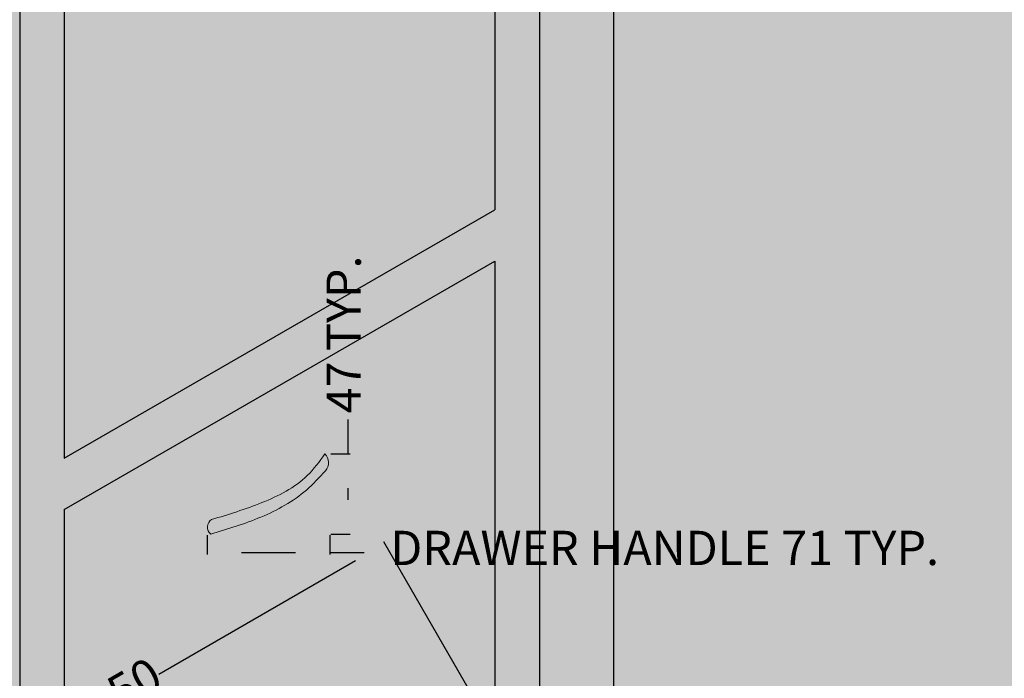
# Model space of a CAD drawing. Units: millimetres. Extents: x 78378 to 86415, y 148682 to 152721.
# Tile 8 of 18: x 79783 to 80358, y 149707 to 150092. Entities that reach past the tile are written whole.
import ezdxf

# ---------------------------------------------------------------- set-up
doc = ezdxf.new("R2010")
doc.units = ezdxf.units.MM
for name, color, linetype, lineweight in [('A-ANNO-DIMS', 2, 'Continuous', 18), ('A-FURN', 4, 'Continuous', 25), ('A-FURN-HRDW', 8, 'Continuous', 18), ('A-FURN-PATT', 32, 'Continuous', 13)]:
    doc.layers.add(name, color=color, linetype=linetype, lineweight=lineweight)
doc.styles.get("Standard").update_dxf_attribs({"font": 'arial.ttf'})
doc.dimstyles.new('ISO-25', dxfattribs={"dimtxt": 20, "dimasz": 20, "dimexe": 1.25, "dimexo": 0.625, "dimtad": 0, "dimdec": 1, "dimtxsty": 'Standard', "dimcen": 2.5, "dimadec": 0, "dimazin": 0, "dimtfac": 1, "dimtdec": 1, "dimtmove": 0, "dimatfit": 3, "dimfxl": 1, "dimarcsym": 0})

# ---------------------------------------------------------------- blocks, each defined once
blk = doc.blocks.new('HANDLE-DRAWER')
for centre, radius, start, end in [((63.38622997708444, 41.62154367045149), 7.231969022595942, 319.3237562697811, 44.69265733271547), ((5.163435732683865, 4.025219173752702), 5.172557027146686, 122.0794663418697, 231.0916038547452)]:
    blk.add_arc(centre, radius, start, end)
for points, knots in [([(2.416316796850878, 8.407990414794767), (12.22361058796001, 11.4080339887645), (31.81170594566225, 17.4000171857454), (55.97206586949582, 29.46692429189343), (65.30177131113433, 42.2784439569471), (68.52736162004294, 46.70781355843064)], [0, 0, 0, 0, 30.92804236988506, 61.77253950703249, 78.07166049105084, 78.07166049105084, 78.07166049105084, 78.07166049105084]), ([(1.914671141596045, 0.0001881390053313), (11.78696018195832, 2.942018891461464), (31.50487046795086, 8.817733694416148), (54.70585002572761, 21.54120260495396), (65.2835446695137, 33.01612223177024), (68.87098889380286, 36.90786192796077)], [0, 0, 0, 0, 30.92804236988506, 61.77253950704738, 77.60214595393334, 77.60214595393334, 77.60214595393334, 77.60214595393334])]:
    blk.add_open_spline(points, degree=3, knots=knots)
blk = doc.blocks.new('*D12')
at = {"layer": 'A-ANNO-DIMS', "color": 0, "lineweight": -2, "transparency": 16777216}
for p, q in [((79892.72448662344, 149790.980188139), (79892.72448662344, 149779.6412546455)), ((79964.1507099133, 149790.980188139), (79964.1507099133, 149779.6412546455)), ((79912.72448662344, 149780.8912546455), (79944.1507099133, 149780.8912546455)), ((79964.1507099133, 149780.8912546455), (79984.1507099133, 149780.8912546455))]:
    blk.add_line(p, q, dxfattribs=at)
at = {"layer": 'A-ANNO-DIMS', "color": 0, "transparency": 16777216}
for points in [[(79912.72448662344, 149784.2245879789), (79912.72448662344, 149777.5579213122), (79892.72448662344, 149780.8912546455)], [(79944.1507099133, 149784.2245879789), (79944.1507099133, 149777.5579213122), (79964.1507099133, 149780.8912546455)]]:
    blk.add_solid(points, dxfattribs=at)
at = {"layer": 'Defpoints', "color": 0, "transparency": 16777216}
for p in [(79892.72448662344, 149791.605188139), (79964.1507099133, 149791.605188139), (79964.1507099133, 149780.8912546455)]:
    blk.add_point(p, dxfattribs=at)
at = {"layer": 'A-ANNO-DIMS', "color": 0, "transparency": 16777216, "insert": (80159.47557348765, 149780.8912546455), "char_height": 20, "attachment_point": 5}
blk.add_mtext('DRAWER HANDLE 71 TYP.', dxfattribs=at)
blk = doc.blocks.new('*D13')
at = {"layer": 'A-ANNO-DIMS', "color": 0, "lineweight": -2, "transparency": 16777216}
for p, q in [((79974.86464340684, 149838.3128135585), (79974.86464340684, 149858.3128135585)), ((79964.77570991333, 149838.3128135585), (79976.11464340684, 149838.3128135585)), ((79974.86464340684, 149811.6051881391), (79974.86464340684, 149818.3128135585)), ((79964.77570991333, 149791.605188139), (79976.11464340684, 149791.605188139))]:
    blk.add_line(p, q, dxfattribs=at)
at = {"layer": 'A-ANNO-DIMS', "color": 0, "transparency": 16777216}
for points in [[(79971.5313100735, 149818.3128135585), (79978.19797674016, 149818.3128135585), (79974.86464340684, 149838.3128135585)], [(79971.5313100735, 149811.6051881391), (79978.19797674016, 149811.6051881391), (79974.86464340684, 149791.605188139)]]:
    blk.add_solid(points, dxfattribs=at)
at = {"layer": 'Defpoints', "color": 0, "transparency": 16777216}
for p in [(79964.15070991333, 149838.3128135585), (79974.86464340684, 149838.3128135585), (79964.15070991333, 149791.605188139)]:
    blk.add_point(p, dxfattribs=at)
at = {"layer": 'A-ANNO-DIMS', "color": 0, "transparency": 16777216, "insert": (79974.86464340687, 149908.0169404343), "char_height": 20, "attachment_point": 5, "rotation": 90}
blk.add_mtext('47 TYP.', dxfattribs=at)
blk = doc.blocks.new('*D22')
at = {"layer": 'A-ANNO-DIMS', "color": 0, "lineweight": -2, "transparency": 16777216}
for p, q in [((80086.091702, 149630.5489088773), (79995.77920202748, 149786.9747473883)), ((79979.08369395178, 149775.8922156335), (79864.48965899751, 149709.7313187051)), ((79710.61581902203, 149620.892215774), (79825.2098539763, 149687.0531127024)), ((79782.98281099998, 149455.5489088774), (79692.67031094636, 149611.9747475287))]:
    blk.add_line(p, q, dxfattribs=at)
at = {"layer": 'A-ANNO-DIMS', "color": 0, "transparency": 16777216}
for points in [[(79977.41702728512, 149778.7789669795), (79980.75036061846, 149773.0054642876), (79996.40420202748, 149785.8922156335)], [(79708.94915235537, 149623.7789671199), (79712.28248568872, 149618.005464428), (79693.29531094636, 149610.892215774)]]:
    blk.add_solid(points, dxfattribs=at)
at = {"layer": 'Defpoints', "color": 0, "transparency": 16777216}
for p in [(79996.40420202748, 149785.8922156335), (80086.404202, 149630.007643), (79783.29531099998, 149455.007643)]:
    blk.add_point(p, dxfattribs=at)
at = {"layer": 'A-ANNO-DIMS', "color": 0, "transparency": 16777216, "insert": (79844.84975648689, 149698.3922157038), "char_height": 20, "attachment_point": 5, "rotation": 30.000000000013433}
blk.add_mtext('350', dxfattribs=at)
blk = doc.blocks.new('*D32')
at = {"layer": 'A-ANNO-DIMS', "color": 0, "lineweight": -2, "transparency": 16777216}
for p, q in [((80086.404202, 150459.382643), (80086.404202, 148693.757643)), ((80692.621985, 150459.382643), (80692.621985, 148693.757643)), ((80106.404202, 148695.007643), (80355.19095843862, 148695.007643)), ((80672.621985, 148695.007643), (80423.8352285614, 148695.007643))]:
    blk.add_line(p, q, dxfattribs=at)
at = {"layer": 'A-ANNO-DIMS', "color": 0, "transparency": 16777216}
for points in [[(80106.404202, 148698.3409763333), (80106.404202, 148691.6743096666), (80086.404202, 148695.007643)], [(80672.621985, 148698.3409763333), (80672.621985, 148691.6743096666), (80692.621985, 148695.007643)]]:
    blk.add_solid(points, dxfattribs=at)
at = {"layer": 'Defpoints', "color": 0, "transparency": 16777216}
for p in [(80086.404202, 150460.007643), (80692.621985, 150460.007643), (80692.621985, 148695.007643)]:
    blk.add_point(p, dxfattribs=at)
at = {"layer": 'A-ANNO-DIMS', "color": 0, "transparency": 16777216, "insert": (80389.5130935, 148695.007643), "char_height": 20, "attachment_point": 5}
blk.add_mtext('606.2', dxfattribs=at)

msp = doc.modelspace()

# ---------------------------------------------------------------- hatches: boundary and pattern name
at = {"layer": 'A-FURN-PATT'}
h = msp.add_hatch(color=256, dxfattribs=at)
h.dxf.hatch_style = 1
h.paths.add_polyline_path([(80389.81355980314, 150935.1811176149), (80389.51309381555, 151105.0076434962), (80164.3464888316, 151105.0076434962), (79904.53886769625, 150955.0076434962), (79433.58476952511, 150683.1021681411), (79459.41281351625, 150662.3818050495), (79243.9048024148, 150537.9581968276), (79160.4069246431, 150518.167363956), (78839.3276210414, 150320.0076434962), (78579.51999990609, 150470.0076434961), (78570.85974586825, 150475.0076434961), (78570.85974586825, 150465.0076434962), (78570.85974586825, 149885.0076434961)])
h.paths.add_polyline_path([(80086.40420249099, 150460.0076434961), (79826.59658135568, 150610.0076434961), (78570.85974586825, 149885.0076434961), (78830.66736700358, 149735.0076434961)])
h.paths.add_polyline_path([(79540.80006404899, 150161.0556565937), (79217.39666007676, 149974.3386142535), (78980.9165707482, 150110.8704574853), (79304.31997472048, 150297.5874998256)], flags=16)
h.paths.add_polyline_path([(79506.15904789761, 150161.0556565937), (79217.39666007677, 149994.3386142535), (79015.55758689957, 150110.8704574853), (79304.31997472048, 150277.5874998256)], flags=0)
edge = h.paths.add_edge_path(flags=0)
edge.add_arc((79247.8635885932, 150177.154059363), 137.979927152229, 256.0025927560106, 293.5594108656914)
edge.add_arc((79240.76712928673, 150078.260535577), 68.08549769177299, 336.0991039681863, 387.369687653981)
edge.add_ellipse((79258.3073696606, 150109.4851683714), major_axis=(-42.62344506003415, -1.659142297571932), ratio=0.1604284291443649, start_angle=0, end_angle=179.0977278657225, ccw=False)
edge.add_arc((79285.21118690472, 150074.2509041072), 77.20964330046426, 155.1233103751286, 203.6557939001038)
edge = h.paths.add_edge_path(flags=0)
edge.add_ellipse((79258.69578401413, 150110.8297486024), major_axis=(-42.62344506003415, -1.659142297571932), ratio=0.1604284291443649, start_angle=350.6039411592706, end_angle=356.2289762200799)
edge.add_line((79219.16897707367, 150111.8937051806), (79218.32684768032, 150109.4140931549))
edge.add_arc((79262.46751974897, 150032.9602064517), 88.28134413732826, 112.39312291994881, 119.99999999999571, ccw=False)
h.paths.add_polyline_path([(79287.06250338514, 150086.9702731333, -0.247702064009433), (79288.19674658246, 150077.2955427019, -0.3904765126137986), (79265.47309673205, 150072.5437639662, -0.4872615262363024), (79264.07897218876, 150082.3768585209, 0.3956043262328261)], flags=0)
h.paths.add_polyline_path([(80389.51309381556, 150935.0076434961), (79826.59658135568, 150610.0076434961), (80086.40420249099, 150460.0076434961), (80692.6219851401, 150460.0076434961), (80952.42960627541, 150610.0076434961)])
edge = h.paths.add_edge_path(flags=16)
edge.add_ellipse((80392.44658491029, 150825.6009587087), major_axis=(-133.0756756189512, 7.721978101297283), ratio=0.424499569836956, start_angle=0, end_angle=360)
edge = h.paths.add_edge_path(flags=0)
edge.add_spline(control_points=[(80269.35411604258, 150832.7436415815), (80269.29193278665, 150831.6720147667), (80269.35031475963, 150830.592249842), (80269.73411879689, 150828.3360718096), (80270.06118209881, 150827.1586823489), (80271.04613754865, 150824.6748448987), (80271.70517726007, 150823.3691586005), (80273.40612032128, 150820.6503360826), (80274.44810410585, 150819.2381263036), (80276.93657810257, 150816.3508564802), (80278.3827638828, 150814.8762414973), (80282.58575216534, 150811.0913237019), (80285.62609899955, 150808.7701423959), (80292.60313446997, 150804.2267034199), (80296.53882829295, 150802.0041234762), (80305.19495220963, 150797.7581273222), (80309.91505114386, 150795.7343743789), (80320.0111596611, 150791.9599857595), (80325.38703862559, 150790.2091628441), (80339.21624322617, 150786.3149836253), (80347.95776464436, 150784.3563224224), (80366.06785395242, 150781.2568288573), (80375.43585590576, 150780.1158444778), (80394.309330179, 150778.7158311894), (80403.81420373028, 150778.4568170495), (80422.465596717, 150778.8319300563), (80431.61154730739, 150779.4662025667), (80449.06079653747, 150781.5837654722), (80457.36359407243, 150783.0675039467), (80472.6698529301, 150786.7766095128), (80479.67258750588, 150789.0032721294), (80490.18936031369, 150793.2813222805), (80494.12675567923, 150795.1967122277), (80501.0145611878, 150799.188512515), (80503.9631522054, 150801.2651387212), (80508.20659370373, 150804.9015163823), (80509.7300059309, 150806.4609393726), (80512.19955536906, 150809.4942049083), (80513.14558327098, 150810.9657349426), (80514.42909982229, 150813.5430698013), (80514.84355071915, 150814.6688389962), (80515.39838138374, 150816.8624682529), (80515.5404646545, 150817.9315158847), (80515.58008082317, 150820.0980035506), (80515.47732053277, 150821.197772811), (80514.99049560675, 150823.5061778107), (80514.6046629432, 150824.7154201442), (80513.48543938114, 150827.2641302181), (80512.7510921682, 150828.6026612985), (80510.88722780815, 150831.3808578872), (80509.75776214547, 150832.8196480674), (80507.0873051963, 150835.7513330261), (80505.5466409065, 150837.243857375), (80501.06238832264, 150841.0944478958), (80497.8199298022, 150843.4575549534), (80490.4173793454, 150848.0619874995), (80486.25822277585, 150850.3037143823), (80477.14480578042, 150854.5642972019), (80472.19085006021, 150856.583496544), (80461.6274878137, 150860.3244857693), (80456.01820904585, 150862.0464562905), (80441.73317330678, 150865.8126742317), (80432.78853232553, 150867.6675482482), (80414.33909310326, 150870.5316780972), (80404.8348928345, 150871.5410542788), (80385.7706775062, 150872.6572210053), (80376.21128671143, 150872.7639759942), (80357.54439280283, 150872.0728395342), (80348.43747055416, 150871.27476178), (80331.16822413795, 150868.8299635098), (80323.00642023917, 150867.1826714935), (80309.47200145545, 150863.5363064667), (80303.8627990537, 150861.6592748057), (80293.8018064812, 150857.5400855607), (80289.35122989668, 150855.2968623192), (80282.77569843757, 150851.2345481044), (80280.34726566746, 150849.4578867352), (80276.26060564672, 150845.9127204516), (80274.60404284154, 150844.1457946164), (80272.31573199967, 150841.1242619346), (80271.53575166185, 150839.8453762844), (80270.34961441216, 150837.3878672019), (80269.94168426798, 150836.2101260174), (80269.5065140611, 150834.2814629481), (80269.3988329965, 150833.5142652193), (80269.35411604258, 150832.7436415815)], knot_values=[0, 0, 0, 0, 0.0975004598125087, 0.0975004598125087, 0.1950009196250173, 0.1950009196250173, 0.2925013794375259, 0.2925013794375259, 0.3900018392500346, 0.3900018392500346, 0.4875022990625432, 0.4875022990625432, 0.6388032241337034, 0.6388032241337034, 0.7901041492048636, 0.7901041492048636, 0.9414050742760238, 0.9414050742760238, 1.092705999347184, 1.092705999347184, 1.312817101002443, 1.312817101002443, 1.532928202657702, 1.532928202657702, 1.753039304312961, 1.753039304312961, 1.973150405968221, 1.973150405968221, 2.19326150762348, 2.19326150762348, 2.413372609278739, 2.413372609278739, 2.569860632934037, 2.569860632934037, 2.726348656589336, 2.726348656589336, 2.844186581547077, 2.844186581547077, 2.962024506504818, 2.962024506504818, 3.060233875946405, 3.060233875946405, 3.158443245387991, 3.158443245387991, 3.256652614829578, 3.256652614829578, 3.354861984271164, 3.354861984271164, 3.453071353712751, 3.453071353712751, 3.551280723154337, 3.551280723154337, 3.649490092595923, 3.649490092595923, 3.803927730406353, 3.803927730406353, 3.958365368216782, 3.958365368216782, 4.112803006027212, 4.112803006027212, 4.267240643837642, 4.267240643837642, 4.489203494974081, 4.489203494974081, 4.711166346110521, 4.711166346110521, 4.93312919724696, 4.93312919724696, 5.155092048383399, 5.155092048383399, 5.377054899519838, 5.377054899519838, 5.557853608626545, 5.557853608626545, 5.738652317733252, 5.738652317733252, 5.872395555677483, 5.872395555677483, 6.006138793621714, 6.006138793621714, 6.109604996023907, 6.109604996023907, 6.2130711984261, 6.2130711984261, 6.283185307179586, 6.283185307179586, 6.283185307179586, 6.283185307179586], degree=3, periodic=0)
edge = h.paths.add_edge_path(flags=0)
edge.add_ellipse((80392.446576265, 150825.6009639553), major_axis=(-101.8397670786795, 3.392257208815831), ratio=0.403492477068114, start_angle=0, end_angle=360)
edge = h.paths.add_edge_path(flags=0)
edge.add_ellipse((80391.1657165424, 150858.3745518381), major_axis=(9.088237780547283, -0.67334552975693), ratio=0.3513541290445306, start_angle=0, end_angle=360)
h.paths.add_polyline_path([(80952.42960627541, 150610.0076434961), (80692.62198514014, 150460.0076434962), (81361.23421645904, 150073.9841917607), (81649.96279182703, 150052.7286159431), (81766.49348583283, 150120.0076434961), (81766.49348583283, 150140.0076434961), (81564.90245463562, 150256.396279624), (81564.88840704803, 150096.1962601479), (81538.90760017018, 150111.1962859926), (81538.92165266915, 150271.3963026331)])
h.paths.add_polyline_path([(81539.035680894, 151571.3304684069), (80867.77935513339, 151958.88048878), (80867.77935513337, 151618.8804887802), (81498.02561065964, 151255.0076434964), (81498.02561065964, 150905.0076434961), (81238.21798952435, 150755.0076434961), (81538.94884401507, 150581.3806037023)])
h.paths.add_polyline_path([(81766.49348583283, 151440.0076434962), (81565.01644300755, 151556.3304684069), (81564.92963647815, 150566.38058618), (81766.49348583283, 150450.0076434962)])
edge = h.paths.add_edge_path()
edge.add_line((81564.92963647815, 150566.38058618), (81564.9136990684, 150384.628856009))
edge.add_ellipse((81552.13037602534, 150358.5718270642), major_axis=(52.62721254190076, 3.506026927036754), ratio=0.4958990548584225, start_angle=367.51697565131457, end_angle=420.0564685523974, ccw=False)
edge.add_ellipse((81552.13037602534, 150358.5718270642), major_axis=(52.62721254190076, 3.506026927036754), ratio=0.4958990548584225, start_angle=351.72974196033346, end_angle=367.51697565131457, ccw=False)
edge.add_ellipse((81552.13037602534, 150345.5015529042), major_axis=(52.62721254190076, 3.506026927036754), ratio=0.4958990548584225, start_angle=352.51169489415116, end_angle=366.30060915387577, ccw=False)
edge.add_line((81603.4463374456, 150342.2038825707), (81603.50642755294, 150340.4474978293))
edge.add_ellipse((81552.13037602534, 150332.1280359686), major_axis=(52.62721254190076, 3.506026927036754), ratio=0.4958990548584225, start_angle=353.6729654395227, end_angle=365.38679972494066, ccw=False)
edge.add_ellipse((81552.13037602534, 150332.1280359686), major_axis=(52.62721254190076, 3.506026927036754), ratio=0.4958990548584225, start_angle=350.9388331002564, end_angle=353.6729654395227)
edge.add_line((81603.86882368504, 150329.8549549892), (81604.0441546891, 150324.7301729966))
edge.add_ellipse((81552.13037602534, 150317.7418284518), major_axis=(52.62721254190076, 3.506026927036754), ratio=0.4958990548584225, start_angle=355.21767463173103, end_angle=363.85533637812415, ccw=False)
edge.add_ellipse((81552.13037602534, 150317.7418284518), major_axis=(52.62721254190076, 3.506026927036754), ratio=0.4958990548584225, start_angle=341.3250873036158, end_angle=355.21767463173103, ccw=False)
edge.add_ellipse((81552.13037602534, 150317.7418284518), major_axis=(52.62721254190076, 3.506026927036754), ratio=0.4958990548584225, start_angle=293.4661701367695, end_angle=341.3250873036158, ccw=False)
edge.add_line((81564.90566138821, 150292.9663898651), (81564.90245463562, 150256.396279624))
edge.add_line((81564.90245463562, 150256.396279624), (81766.49348583283, 150140.0076434961))
edge.add_line((81766.49348583283, 150140.0076434961), (81766.49348583283, 150450.0076434962))
edge.add_line((81766.49348583283, 150450.0076434962), (81564.92963647815, 150566.38058618))
h.paths.add_polyline_path([(81525.57129610774, 150321.5980043728), (81526.59848255829, 150321.3069082928), (81528.6771290606, 150320.947049251)])
h.paths.add_polyline_path([(81512.79027333307, 150326.1128631878), (81514.50580755486, 150325.38873887), (81512.53799543541, 150326.2678422534)])
h.paths.add_polyline_path([(81533.21477271736, 150320.1614841748), (81534.69519629495, 150319.9051905676), (81536.59953044976, 150319.755668921)])
h.paths.add_polyline_path([(81518.62200466282, 150323.6512984944), (81519.22704244989, 150323.3959129888), (81521.28902816366, 150322.8115634216)])
h.paths.add_polyline_path([(81501.21834684846, 150336.259909523), (81500.35429342867, 150338.133928838), (81499.78149159584, 150340.0493926212), (81499.50316348342, 150341.9955259773), (81499.50316348343, 150343.7256661642), (81499.75838934928, 150345.5905095656), (81500.27655404429, 150347.4549063508), (81501.05505607055, 150349.3094961287), (81501.09670215519, 150349.3936770376), (81501.13888119749, 150349.4778172982), (81500.99777251929, 150349.749637304), (81500.86282558287, 150350.0225204294), (81499.50316348342, 150355.0658001372), (81499.95910976747, 150359.5002298216), (81501.89819062682, 150363.9082666975), (81505.26528150582, 150368.1645982632), (81509.96466211145, 150372.148224724), (81515.86273756725, 150375.7458987972), (81522.79183627458, 150378.8553451273), (81530.55497651099, 150381.3881677888), (81538.93146626501, 150383.2723632221), (81538.94884401507, 150581.3806037023), (80632.00020687521, 151105.0076434962), (80389.51309381555, 151105.0076434962), (80389.81417426979, 150934.8338146148), (80952.42960627541, 150610.0076434961), (81538.92165266915, 150271.3963026331), (81538.92343538092, 150291.719410528), (81538.87516273293, 150291.7210326448), (81530.1914951021, 150292.8238998863), (81522.18015347481, 150294.6903872688), (81515.08664870211, 150297.2632955209), (81509.86347084012, 150299.9959433281), (81505.6084410237, 150303.1350709547), (81502.41902318504, 150306.608774857), (81500.3682727948, 150310.3374878268), (81499.50316348343, 150314.2358015248), (81499.50316348343, 150315.9659417118), (81499.82059494797, 150318.1159244827), (81500.4869945128, 150320.2634115907), (81501.49791650465, 150322.3940767571), (81500.48699451279, 150324.4232810552), (81499.82059494796, 150326.50388518), (81499.50316348343, 150328.6220090417), (81499.50316348343, 150330.3521492286), (81499.78149159584, 150332.3262168982), (81500.35429342862, 150334.2991697576)])
h = msp.add_hatch(color=256, dxfattribs=at)
h.dxf.hatch_style = 1
h.paths.add_polyline_path([(80692.6219851401, 150440.0076434962), (80086.40420249102, 150440.0076434962), (80086.40420249104, 149630.0076434962), (80692.62198514013, 149614.0076434961)])
h.paths.add_polyline_path([(80293.42096661613, 150335.1041026971, -0.693913746763918), (80505.02836664302, 150344.7159628166, -0.266337996674739), (80649.3207149509, 150178.1038520679), (80649.32071495091, 149665.150500639), (80129.70547268025, 149678.8647863533), (80129.70547268025, 150178.1038520678, -0.257326206066023)], flags=16)
h.paths.add_polyline_path([(80060.4234403775, 150384.3023755343), (79809.27607328002, 150239.3023755343), (79809.27607328001, 150141.6366131478), (80060.4234403775, 150286.6366131478)])
h.paths.add_polyline_path([(80086.40420249102, 150399.3023755343), (80086.40420249102, 150440.0076434961), (79783.29531116647, 150265.0076434962), (79783.29531116647, 150224.3023755343)])
edge = h.paths.add_edge_path(flags=16)
edge.add_arc((79946.63023943067, 150348.8762810125), 10.76362312575662, -18.381796908867102, 28.033199430885304, ccw=False)
edge.add_spline(control_points=[(79956.8446621052, 150345.4819987291), (79949.48615957417, 150336.2391268092), (79933.85278209679, 150316.6023454005), (79908.95072794275, 150312.561963116), (79895.76986639632, 150310.4233556278)], knot_values=[0, 0, 0, 0, 34.22568399180864, 72.71357657474474, 72.71357657474474, 72.71357657474474, 72.71357657474474], degree=3, periodic=0)
edge.add_arc((79899.38686741845, 150314.0155032977), 5.097668219542309, 123.6496152582665, 224.8024750763005, ccw=False)
edge.add_spline(control_points=[(79896.56218517898, 150318.2590149947), (79909.86104355381, 150320.2802713686), (79934.78207045459, 150324.0679487052), (79949.34122059586, 150344.4361083294), (79956.13102493295, 150353.9350019607)], knot_values=[0, 0, 0, 0, 38.48789258293611, 72.12331911350849, 72.12331911350849, 72.12331911350849, 72.12331911350849], degree=3, periodic=0)
h.paths.add_polyline_path([(80086.40420249102, 150399.3023755343), (80060.4234403775, 150384.3023755343), (80060.4234403775, 150286.6366131478), (80086.40420249102, 150301.6366131477)], flags=17)
h.paths.add_polyline_path([(79809.27607328002, 150239.3023755343), (79783.29531116647, 150224.3023755343), (79783.29531116647, 150126.6366131478), (79809.27607328001, 150141.6366131478)])
h = msp.add_hatch(color=256, dxfattribs=at)
h.dxf.hatch_style = 1
h.paths.add_polyline_path([(80060.4234403775, 150256.6366131478), (79809.27607328001, 150111.6366131478), (79809.27607328001, 149835.822128322), (80060.4234403775, 149980.822128322)])
edge = h.paths.add_edge_path(flags=16)
edge.add_arc((79897.98743573268, 150103.5556037615), 5.172557027142873, 122.07946634250479, 231.0916038546426, ccw=False)
edge.add_spline(control_points=[(79895.24031679684, 150107.9383750026), (79905.04761058795, 150110.9384185765), (79924.63570594566, 150116.9304017735), (79948.79606586948, 150128.9973088797), (79958.12577131113, 150141.8088285447), (79961.35136162004, 150146.2381981462)], knot_values=[0, 0, 0, 0, 30.92804236988506, 61.77253950703249, 78.07166049105084, 78.07166049105084, 78.07166049105084, 78.07166049105084], degree=3, periodic=0)
edge.add_arc((79956.21022997708, 150141.1519282582), 7.231969022599169, -40.6762437318896, 44.692657332507395, ccw=False)
edge.add_spline(control_points=[(79961.6949888938, 150136.4382465157), (79958.1075446695, 150132.5465068195), (79947.5298500257, 150121.0715871927), (79924.32887046793, 150108.3481182822), (79904.61096018193, 150102.4724034792), (79894.73867114159, 150099.5305727268)], knot_values=[0, 0, 0, 0, 15.82960644688596, 46.67410358404827, 77.60214595393333, 77.60214595393333, 77.60214595393333, 77.60214595393333], degree=3, periodic=0)
h.paths.add_polyline_path([(80060.4234403775, 149950.8221283219), (79809.27607328001, 149805.822128322), (79809.27607328001, 149500.0076434962), (80060.42344037753, 149645.0076434962)])
h.paths.add_polyline_path([(80649.3207149509, 150178.1038520679, 0.2663379966747387), (80505.02836664302, 150344.7159628166, 0.6939137467639167), (80293.42096661613, 150335.1041026971, 0.2573262060660234), (80129.70547268025, 150178.1038520678), (80129.70547268025, 149678.8647863533), (80649.32071495091, 149665.150500639)])
h = msp.add_hatch(color=256, dxfattribs=at)
h.dxf.hatch_style = 1
h.paths.add_polyline_path([(79765.97480309076, 149445.0076434962), (79765.97480309078, 149603.6183766167), (79275.17610351968, 149320.2556153015), (79275.17610351968, 149161.6448821809), (79350.28260927423, 149205.0076434961)])
edge = h.paths.add_edge_path(flags=16)
edge.add_arc((79507.24398653943, 149406.7325176549), 51.45725872682493, 189.4892033869566, 208.9818028088169, ccw=False)
edge.add_spline(control_points=[(79456.49083369225, 149398.249183891), (79490.7805017203, 149406.8496318209), (79544.66821365236, 149420.3656116243), (79585.61673544894, 149461.098953088), (79597.20784070941, 149478.6256589295), (79597.88663588953, 149479.65205315)], knot_values=[0, 0, 0, 0, 103.8711517509291, 163.2380546532031, 166.9309452742424, 166.9309452742424, 166.9309452742424, 166.9309452742424], degree=3, periodic=0)
edge.add_arc((79598.46803720549, 149470.6288681557), 9.041896644556108, -55.21570256624602, 93.686708761847, ccw=False)
edge.add_spline(control_points=[(79603.62633526741, 149463.2027079073), (79602.94754008728, 149462.1763136868), (79591.3564348269, 149444.6496078453), (79550.40791303018, 149403.9162663817), (79496.52020109817, 149390.4002865783), (79462.23053307013, 149381.7998386483)], knot_values=[0, 0, 0, 0, 3.692890621039242, 63.05979352331328, 166.9309452742424, 166.9309452742424, 166.9309452742424, 166.9309452742424], degree=3, periodic=0)
h.paths.add_polyline_path([(80060.4234403775, 149980.822128322), (80060.4234403775, 150256.6366131478), (79809.27607328001, 150111.6366131478), (79809.27607328001, 149835.822128322)], flags=0)
edge = h.paths.add_edge_path(flags=0)
edge.add_arc((79897.98743573268, 150103.5556037615), 5.172557027142874, 122.07946634250479, 231.0916038545171, ccw=False)
edge.add_spline(control_points=[(79895.24031679684, 150107.9383750026), (79905.04761058795, 150110.9384185765), (79924.63570594566, 150116.9304017735), (79948.79606586948, 150128.9973088797), (79958.12577131113, 150141.8088285447), (79961.35136162004, 150146.2381981462)], knot_values=[0, 0, 0, 0, 30.92804236988506, 61.77253950703249, 78.07166049105084, 78.07166049105084, 78.07166049105084, 78.07166049105084], degree=3, periodic=0)
edge.add_arc((79956.21022997708, 150141.1519282582), 7.231969022599169, -40.6762437318896, 44.692657332507395, ccw=False)
edge.add_spline(control_points=[(79961.6949888938, 150136.4382465157), (79958.1075446695, 150132.5465068195), (79947.5298500257, 150121.0715871927), (79924.32887046793, 150108.3481182822), (79904.61096018193, 150102.4724034792), (79894.73867114159, 150099.5305727268)], knot_values=[0, 0, 0, 0, 15.82960644688596, 46.67410358404827, 77.60214595393333, 77.60214595393333, 77.60214595393333, 77.60214595393333], degree=3, periodic=0)
h.paths.add_polyline_path([(80060.4234403775, 149950.8221283219), (79809.27607328001, 149805.822128322), (79809.27607328001, 149500.0076434962), (80060.42344037753, 149645.0076434962)], flags=0)
edge = h.paths.add_edge_path(flags=0)
edge.add_arc((79897.98743573268, 149795.6302191737), 5.172557027142842, 122.07946634250479, 231.0916038545171, ccw=False)
edge.add_spline(control_points=[(79895.24031679684, 149800.0129904148), (79905.04761058795, 149803.0130339888), (79924.63570594566, 149809.0050171857), (79948.79606586948, 149821.0719242919), (79958.12577131113, 149833.883443957), (79961.35136162004, 149838.3128135584)], knot_values=[0, 0, 0, 0, 30.92804236988506, 61.77253950703249, 78.07166049105084, 78.07166049105084, 78.07166049105084, 78.07166049105084], degree=3, periodic=0)
edge.add_arc((79956.21022997708, 149833.2265436705), 7.231969022599074, -40.6762437318896, 44.692657332507395, ccw=False)
edge.add_spline(control_points=[(79961.6949888938, 149828.5128619279), (79958.1075446695, 149824.6211222318), (79947.5298500257, 149813.1462026049), (79924.32887046793, 149800.4227336944), (79904.61096018193, 149794.5470188914), (79894.73867114159, 149791.605188139)], knot_values=[0, 0, 0, 0, 15.82960644688596, 46.67410358404827, 77.60214595393333, 77.60214595393333, 77.60214595393333, 77.60214595393333], degree=3, periodic=0)
h.paths.add_polyline_path([(80086.40420249102, 150301.6366131477), (79783.29531116647, 150126.6366131478), (79783.29531116645, 149455.0076434962), (80086.40420249104, 149630.0076434962)])
h.paths.add_polyline_path([(79809.27607328001, 150111.6366131478), (80060.4234403775, 150256.6366131478), (80060.4234403775, 149980.822128322), (79809.27607328001, 149835.822128322)], flags=16)
h.paths.add_polyline_path([(80060.4234403775, 149950.8221283219), (80060.42344037753, 149645.0076434962), (79809.27607328001, 149500.0076434962), (79809.27607328001, 149805.822128322)], flags=16)
h = msp.add_hatch(color=256, dxfattribs=at)
h.dxf.hatch_style = 1
h.paths.add_polyline_path([(79765.97480309078, 150214.3023755343), (79275.17610351971, 149930.939614219), (79275.17610351968, 149340.2556153015), (79361.10187436163, 149389.8648822274), (79361.10187436163, 149854.0251874417), (79688.53915659874, 150043.071190484), (79688.53915659874, 149578.9108852697), (79765.97480309078, 149623.6183766168)], flags=0)
h.paths.add_polyline_path([(79616.99747211508, 150064.3357852431, -1), (79579.57778226466, 150064.3357852431, -1)], flags=0)
h.paths.add_polyline_path([(79511.25702160504, 150003.2865076769, -1), (79473.83733175462, 150003.2865076769, -1)], flags=0)
h.paths.add_polyline_path([(79398.61463104078, 149938.2523931624, -1), (79361.19494119036, 149938.2523931624, -1)], flags=0)
h.paths.add_polyline_path([(79688.53915659874, 149578.9108852697), (79667.16069404285, 149674.8368362752), (79401.25237372774, 149521.3145959615), (79361.10187436163, 149389.8648822274)], flags=0)
h.paths.add_polyline_path([(79783.29531116645, 149613.6183766167), (79783.29531116647, 150126.6366131478), (79783.29531116647, 150265.0076434962), (79257.85559544402, 149961.6448821809), (79257.85559544401, 149310.2556153015)])
h.paths.add_polyline_path([(79275.17610351968, 149340.2556153015), (79275.17610351971, 149930.939614219), (79765.97480309078, 150214.3023755343), (79765.97480309078, 149623.6183766168)], flags=16)
h.paths.add_polyline_path([(79361.10187436163, 149389.8648822274), (79361.10187436163, 149854.0251874417), (79688.53915659874, 150043.071190484), (79688.53915659874, 149578.9108852697), (79667.16069404285, 149674.8368362752), (79401.25237372774, 149521.3145959615)], flags=0)
h.paths.add_polyline_path([(79477.90289169294, 149864.6773096294), (79477.90289169294, 149877.6075739832), (79571.78517238796, 149931.8105340146), (79571.78517238796, 149918.8802696608)], flags=0)

# ---------------------------------------------------------------- linework, layer by layer
at = {"layer": 'A-FURN'}
for p, q in [((80086.40420249102, 150460.0076434962), (80086.40420249104, 149630.0076434962)), ((79783.29531116647, 150285.0076434961), (79783.29531116645, 149455.0076434961)), ((80060.4234403775, 150256.6366131478), (80060.4234403775, 149980.822128322)), ((80129.70547268025, 150178.1038520678), (80129.70547268025, 149678.8647863533)), ((79783.29531116647, 150126.6366131478), (79783.29531116645, 149455.0076434962)), ((79809.27607328001, 150111.6366131478), (79809.27607328001, 149835.822128322)), ((79809.27607328001, 149835.822128322), (80060.4234403775, 149980.822128322)), ((79809.27607328001, 149805.822128322), (80060.4234403775, 149950.8221283219)), ((80060.4234403775, 149950.8221283219), (80060.42344037753, 149645.0076434962)), ((79809.27607328001, 149805.822128322), (79809.27607328001, 149500.0076434962))]:
    msp.add_line(p, q, dxfattribs=at)

# ---------------------------------------------------------------- block references
at = {"layer": 'A-FURN-HRDW'}
msp.add_blockref('HANDLE-DRAWER', (79892.824, 149791.605), dxfattribs=at)

# ---------------------------------------------------------------- dimensions: what is measured, and where the dimension line sits
at = {"layer": 'A-ANNO-DIMS'}
dim = msp.add_linear_dim(base=(80692.621985, 148695.007643), p1=(80086.404202, 150460.007643), p2=(80692.621985, 150460.007643), dimstyle='ISO-25', override={"dimdec": 1, "dimlfac": 1, "dimrnd": 0, "dimzin": 0, "dimdsep": 46, "dimlunit": 2}, dxfattribs=at)
dim.commit()
dim.dimension.update_dxf_attribs({"geometry": '*D32', "text_midpoint": (80389.5130935, 148695.007643)})
dim = msp.add_linear_dim(base=(79974.86464340684, 149838.3128135585), p1=(79964.1507099133, 149791.605188139), p2=(79964.1507099133, 149838.3128135585), angle=90, text='<> TYP.', dimstyle='ISO-25', override={"dimdec": 0, "dimrnd": 0, "dimzin": 0, "dimlunit": 2}, dxfattribs=at)
dim.commit()
dim.dimension.update_dxf_attribs({"geometry": '*D13', "text_midpoint": (79974.86464340687, 149908.0169404343)})
dim = msp.add_linear_dim(base=(79964.1507099133, 149780.8912546455), p1=(79892.72448662344, 149791.605188139), p2=(79964.1507099133, 149791.605188139), text='DRAWER HANDLE <> TYP.', dimstyle='ISO-25', override={"dimdec": 0, "dimrnd": 0, "dimzin": 0, "dimlunit": 2}, dxfattribs=at)
dim.commit()
dim.dimension.update_dxf_attribs({"geometry": '*D12', "text_midpoint": (80159.47557348765, 149780.8912546455)})
dim = msp.add_linear_dim(base=(79996.40420202748, 149785.8922156335), p1=(79783.295311, 149455.007643), p2=(80086.404202, 149630.007643), angle=30.00000000001342, dimstyle='ISO-25', override={"dimdec": 0, "dimlfac": 1, "dimrnd": 0, "dimzin": 0, "dimdsep": 46, "dimlunit": 2}, dxfattribs=at)
dim.commit()
dim.dimension.update_dxf_attribs({"geometry": '*D22', "text_midpoint": (79844.84975648689, 149698.3922157038)})

doc.saveas('drawing.dxf')
